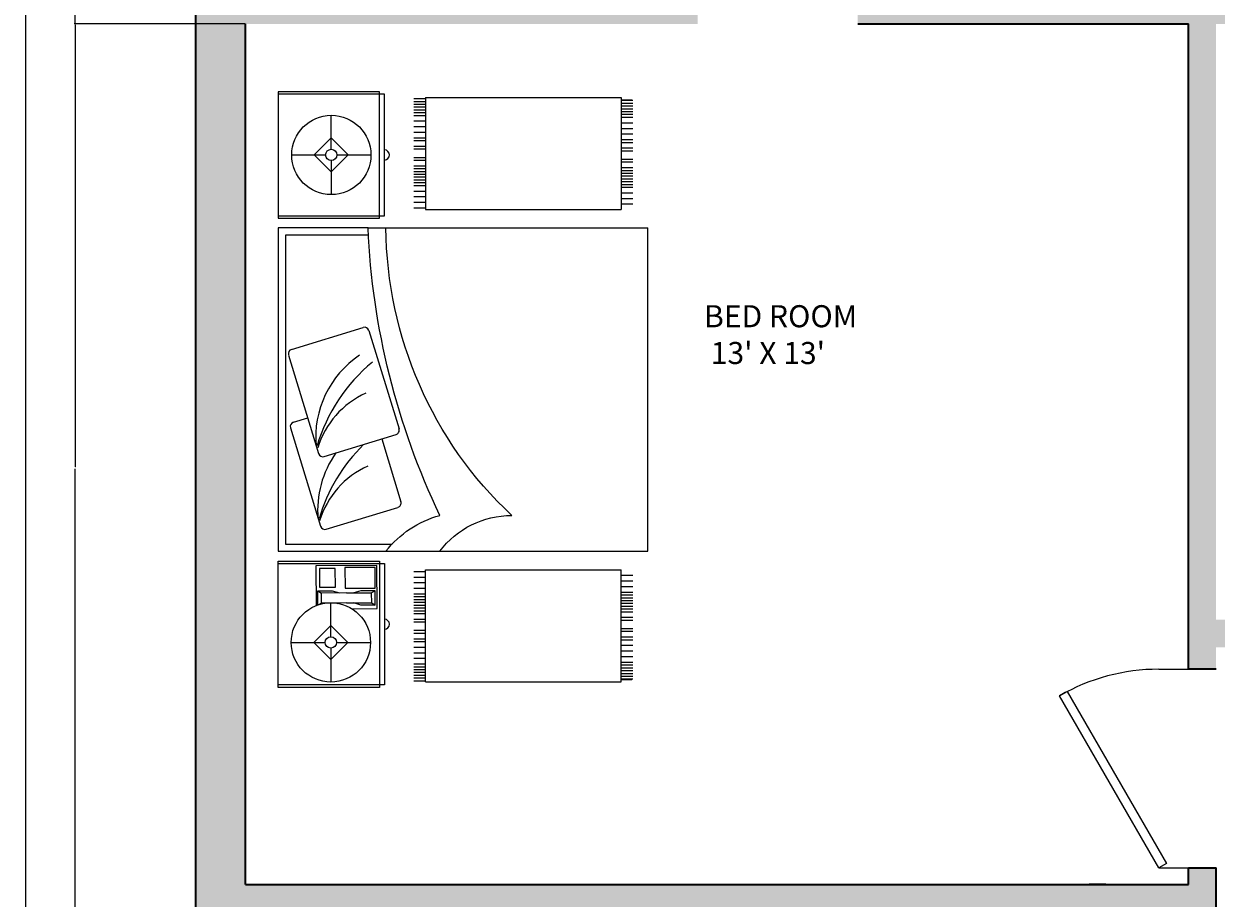
# Model space of a CAD drawing. Units: inches. Extents: x -30 to 437, y -29 to 647.
# Tile 8 of 15: x -30 to 187, y 389 to 548. Entities that reach past the tile are written whole.
import ezdxf

# ---------------------------------------------------------------- set-up
doc = ezdxf.new("R2010")
doc.units = ezdxf.units.IN
doc.header["$MEASUREMENT"] = 0
for name, color, linetype, lineweight in [('A-ANNO-DIMS', 2, 'Continuous', 18), ('A-AREA-IDEN', 7, 'Continuous', 18), ('A-WALL', 7, 'Continuous', 35), ('bedroom', 120, 'Continuous', 18), ('doors', 40, 'Continuous', 25)]:
    doc.layers.add(name, color=color, linetype=linetype, lineweight=lineweight)
doc.layers.add('A-WALL-PATT', color=251, linetype='Continuous', lineweight=13, true_color=0x636466)
doc.styles.get("Standard").update_dxf_attribs({"font": 'arial.ttf'})
doc.dimstyles.get("Standard").update_dxf_attribs({"dimtxt": 0.18, "dimasz": 0.18, "dimexe": 0.18, "dimexo": 0.0625, "dimgap": 0.09, "dimtad": 0, "dimtih": 1, "dimtoh": 1, "dimdec": 4, "dimzin": 0, "dimdsep": 46, "dimtxsty": 'Standard', "dimcen": 0.09, "dimadec": 0, "dimazin": 0, "dimtfac": 1, "dimtdec": 4, "dimtofl": 0, "dimtmove": 0, "dimatfit": 3, "dimfxl": 1, "dimtolj": 1, "dimtzin": 0, "dimarcsym": 0})

# ---------------------------------------------------------------- blocks, each defined once
blk = doc.blocks.new('3')
for p, q in [((185.8665, 224.6766), (185.8665, 225.2363)), ((185.8665, 225.2363), (186.566, 225.2363)), ((185.8805, 224.6487), (185.8805, 225.2363)), ((186.552, 225.2363), (186.552, 224.6487)), ((186.566, 225.2363), (186.566, 224.6766)), ((186.6199, 225.2363), (186.6199, 224.6399)), ((188.4089, 225.2363), (186.6199, 225.2363)), ((188.4089, 224.7393), (188.4089, 225.2363)), ((188.4627, 225.2363), (188.4627, 224.6766)), ((189.1623, 225.2363), (188.4627, 225.2363)), ((188.4767, 225.2363), (188.4767, 224.6486)), ((189.1483, 224.6486), (189.1483, 225.2363)), ((189.1623, 224.6766), (189.1623, 225.2363)), ((186.1157, 225.1643), (186.1157, 224.9763)), ((187.3034, 225.1683), (186.7581, 225.0015)), ((187.7059, 225.1793), (187.1607, 225.0124)), ((187.3344, 225.1518), (187.3586, 225.073)), ((187.737, 225.1628), (187.8585, 224.7657)), ((188.8125, 225.1618), (188.8125, 224.9738)), ((186.0216, 224.9449), (186.1157, 225.0389)), ((186.1157, 225.0389), (186.2097, 224.9449)), ((186.5397, 225.0274), (186.3193, 225.0266)), ((186.3215, 225.0167), (186.4008, 225.017)), ((186.3334, 224.9969), (186.3215, 225.0167)), ((186.3334, 224.9969), (186.389, 224.9971)), ((186.334, 224.858), (186.3334, 224.9969)), ((186.4008, 225.017), (186.389, 224.9971)), ((186.3895, 224.8582), (186.389, 224.9971)), ((186.4008, 225.017), (186.4011, 224.9376)), ((186.5409, 224.6901), (186.5397, 225.0274)), ((188.8125, 225.0365), (188.7185, 224.9424)), ((188.9065, 224.9424), (188.8125, 225.0365)), ((186.0843, 224.9449), (185.8963, 224.9449)), ((186.1157, 224.8509), (186.0216, 224.9449)), ((186.2097, 224.9449), (186.1157, 224.8509)), ((186.147, 224.9449), (186.335, 224.9449)), ((186.4011, 224.9376), (186.3894, 224.8979)), ((186.7416, 224.9704), (186.8631, 224.5734)), ((187.1442, 224.9814), (187.2657, 224.5843)), ((188.7812, 224.9424), (188.5931, 224.9424)), ((188.7185, 224.9424), (188.8125, 224.8484)), ((188.8125, 224.8484), (188.9065, 224.9424)), ((188.8438, 224.9424), (189.0319, 224.9424)), ((186.1157, 224.9136), (186.1157, 224.7256)), ((186.3314, 224.9055), (186.3338, 224.8977)), ((186.334, 224.858), (186.3345, 224.7191)), ((186.3895, 224.8582), (186.39, 224.7193)), ((188.8125, 224.9111), (188.8125, 224.723)), ((186.3023, 224.8297), (186.3029, 224.6892)), ((186.3224, 224.7786), (186.3341, 224.8183)), ((186.4017, 224.7789), (186.3897, 224.8185)), ((186.3227, 224.6992), (186.3224, 224.7786)), ((186.402, 224.6995), (186.4017, 224.7789)), ((187.842, 224.7347), (187.2967, 224.5678)), ((188.4089, 224.7393), (188.4089, 223.1907)), ((186.566, 224.6766), (185.8665, 224.6766)), ((186.3029, 224.6892), (186.5409, 224.6901)), ((186.3345, 224.7191), (186.3227, 224.6992)), ((186.3227, 224.6992), (186.402, 224.6995)), ((186.3345, 224.7191), (186.39, 224.7193)), ((186.402, 224.6995), (186.39, 224.7193)), ((187.2416, 224.6632), (186.8942, 224.5569)), ((188.4627, 224.6766), (189.1623, 224.6766)), ((186.552, 224.6487), (185.8805, 224.6487)), ((186.6199, 224.6399), (186.6199, 223.1907)), ((188.4767, 224.6486), (189.1483, 224.6486)), ((185.904, 224.4849, -0.9094), (185.904, 224.4204, -0.9094)), ((185.9195, 224.4849, -0.9094), (185.9195, 224.4204, -0.9094)), ((185.9195, 224.4849, -0.9094), (185.9195, 224.4204, -0.9094)), ((185.935, 224.4849, -0.9094), (185.935, 224.4204, -0.9094)), ((185.9505, 224.4849, -0.9094), (185.9505, 224.4204, -0.9094)), ((185.966, 224.4849, -0.9094), (185.966, 224.4204, -0.9094)), ((185.9815, 224.4849, -0.9094), (185.9815, 224.4204, -0.9094)), ((185.997, 224.4849, -0.9094), (185.997, 224.4204, -0.9094)), ((186.028, 224.4849, -0.9094), (186.028, 224.4204, -0.9094)), ((186.059, 224.4849, -0.9094), (186.059, 224.4204, -0.9094)), ((186.09, 224.4849, -0.9094), (186.09, 224.4204, -0.9094)), ((186.09, 224.4849, -0.9094), (186.09, 224.4204, -0.9094)), ((186.121, 224.4849, -0.9094), (186.121, 224.4204, -0.9094)), ((186.1365, 224.4849, -0.9094), (186.1365, 224.4204, -0.9094)), ((186.1675, 224.4849, -0.9094), (186.1675, 224.4204, -0.9094)), ((186.183, 224.4849, -0.9094), (186.183, 224.4204, -0.9094)), ((186.2295, 224.4849, -0.9094), (186.2295, 224.4204, -0.9094)), ((186.245, 224.4849, -0.9094), (186.245, 224.4204, -0.9094)), ((186.276, 224.4849, -0.9094), (186.276, 224.4204, -0.9094)), ((186.2915, 224.4849, -0.9094), (186.2915, 224.4204, -0.9094)), ((186.307, 224.4849, -0.9094), (186.307, 224.4204, -0.9094)), ((186.3225, 224.4849, -0.9094), (186.3225, 224.4204, -0.9094)), ((186.338, 224.4849, -0.9094), (186.338, 224.4204, -0.9094)), ((186.3535, 224.4849, -0.9094), (186.3535, 224.4204, -0.9094)), ((186.369, 224.4849, -0.9094), (186.369, 224.4204, -0.9094)), ((186.3845, 224.4849, -0.9094), (186.3845, 224.4204, -0.9094)), ((186.4155, 224.4849, -0.9094), (186.4155, 224.4204, -0.9094)), ((186.4465, 224.4849, -0.9094), (186.4465, 224.4204, -0.9094)), ((186.4775, 224.4849, -0.9094), (186.4775, 224.4204, -0.9094)), ((186.5085, 224.4849, -0.9094), (186.5085, 224.4204, -0.9094)), ((188.5202, 224.4849, -0.9094), (188.5202, 224.4204, -0.9094)), ((188.5512, 224.4849, -0.9094), (188.5512, 224.4204, -0.9094)), ((188.5822, 224.4849, -0.9094), (188.5822, 224.4204, -0.9094)), ((188.6132, 224.4849, -0.9094), (188.6132, 224.4204, -0.9094)), ((188.6442, 224.4849, -0.9094), (188.6442, 224.4204, -0.9094)), ((188.6597, 224.4849, -0.9094), (188.6597, 224.4204, -0.9094)), ((188.6752, 224.4849, -0.9094), (188.6752, 224.4204, -0.9094)), ((188.6907, 224.4849, -0.9094), (188.6907, 224.4204, -0.9094)), ((188.7062, 224.4849, -0.9094), (188.7062, 224.4204, -0.9094)), ((188.7217, 224.4849, -0.9094), (188.7217, 224.4204, -0.9094)), ((188.7372, 224.4849, -0.9094), (188.7372, 224.4204, -0.9094)), ((188.7527, 224.4849, -0.9094), (188.7527, 224.4204, -0.9094)), ((188.7837, 224.4849, -0.9094), (188.7837, 224.4204, -0.9094)), ((188.7992, 224.4849, -0.9094), (188.7992, 224.4204, -0.9094)), ((188.8457, 224.4849, -0.9094), (188.8457, 224.4204, -0.9094)), ((188.8612, 224.4849, -0.9094), (188.8612, 224.4204, -0.9094)), ((188.8922, 224.4849, -0.9094), (188.8922, 224.4204, -0.9094)), ((188.9077, 224.4849, -0.9094), (188.9077, 224.4204, -0.9094)), ((188.9387, 224.4849, -0.9094), (188.9387, 224.4204, -0.9094)), ((188.9387, 224.4849, -0.9094), (188.9387, 224.4204, -0.9094)), ((188.9697, 224.4849, -0.9094), (188.9697, 224.4204, -0.9094)), ((189.0007, 224.4849, -0.9094), (189.0007, 224.4204, -0.9094)), ((189.0317, 224.4849, -0.9094), (189.0317, 224.4204, -0.9094)), ((189.0472, 224.4849, -0.9094), (189.0472, 224.4204, -0.9094)), ((189.0627, 224.4849, -0.9094), (189.0627, 224.4204, -0.9094)), ((189.0782, 224.4849, -0.9094), (189.0782, 224.4204, -0.9094)), ((189.0937, 224.4849, -0.9094), (189.0937, 224.4204, -0.9094)), ((189.1092, 224.4849, -0.9094), (189.1092, 224.4204, -0.9094)), ((189.1092, 224.4849, -0.9094), (189.1092, 224.4204, -0.9094)), ((189.1247, 224.4849, -0.9094), (189.1247, 224.4204, -0.9094)), ((185.8974, 224.4204, -0.9094), (185.8974, 223.3378, -0.9094)), ((185.8974, 224.4204, -0.9094), (186.5174, 224.4204, -0.9094)), ((186.5174, 224.4204, -0.9094), (186.5174, 223.3378, -0.9094)), ((189.1313, 224.4204, -0.9094), (188.5113, 224.4204, -0.9094)), ((188.5113, 224.4204, -0.9094), (188.5113, 223.3378, -0.9094)), ((189.1313, 224.4204, -0.9094), (189.1313, 223.3378, -0.9094)), ((185.8974, 223.3378, -0.9094), (186.5174, 223.3378, -0.9094)), ((185.9114, 223.3378, -0.9094), (185.9114, 223.2789, -0.9094)), ((185.9114, 223.3378, -0.9094), (185.9114, 223.2789, -0.9094)), ((185.9114, 223.3378, -0.9094), (185.9114, 223.2789, -0.9094)), ((185.9138, 223.3378, -0.9094), (185.9138, 223.2732, -0.9094)), ((185.9293, 223.3378, -0.9094), (185.9293, 223.2732, -0.9094)), ((185.9293, 223.3378, -0.9094), (185.9293, 223.2732, -0.9094)), ((185.9448, 223.3378, -0.9094), (185.9448, 223.2732, -0.9094)), ((185.9603, 223.3378, -0.9094), (185.9603, 223.2732, -0.9094)), ((185.9758, 223.3378, -0.9094), (185.9758, 223.2732, -0.9094)), ((185.9913, 223.3378, -0.9094), (185.9913, 223.2732, -0.9094)), ((186.0068, 223.3378, -0.9094), (186.0068, 223.2732, -0.9094)), ((186.0378, 223.3378, -0.9094), (186.0378, 223.2732, -0.9094)), ((186.0688, 223.3378, -0.9094), (186.0688, 223.2732, -0.9094)), ((186.0998, 223.3378, -0.9094), (186.0998, 223.2732, -0.9094)), ((186.0998, 223.3378, -0.9094), (186.0998, 223.2732, -0.9094)), ((186.1308, 223.3378, -0.9094), (186.1308, 223.2732, -0.9094)), ((186.1463, 223.3378, -0.9094), (186.1463, 223.2732, -0.9094)), ((186.1773, 223.3378, -0.9094), (186.1773, 223.2732, -0.9094)), ((186.1928, 223.3378, -0.9094), (186.1928, 223.2732, -0.9094)), ((186.2393, 223.3378, -0.9094), (186.2393, 223.2732, -0.9094)), ((186.2548, 223.3378, -0.9094), (186.2548, 223.2732, -0.9094)), ((186.2858, 223.3378, -0.9094), (186.2858, 223.2732, -0.9094)), ((186.3013, 223.3378, -0.9094), (186.3013, 223.2732, -0.9094)), ((186.3168, 223.3378, -0.9094), (186.3168, 223.2732, -0.9094)), ((186.3323, 223.3378, -0.9094), (186.3323, 223.2732, -0.9094)), ((186.3478, 223.3378, -0.9094), (186.3478, 223.2732, -0.9094)), ((186.3633, 223.3378, -0.9094), (186.3633, 223.2732, -0.9094)), ((186.3788, 223.3378, -0.9094), (186.3788, 223.2732, -0.9094)), ((186.3943, 223.3378, -0.9094), (186.3943, 223.2732, -0.9094)), ((186.4253, 223.3378, -0.9094), (186.4253, 223.2732, -0.9094)), ((186.4563, 223.3378, -0.9094), (186.4563, 223.2732, -0.9094)), ((186.4873, 223.3378, -0.9094), (186.4873, 223.2732, -0.9094)), ((189.1313, 223.3378, -0.9094), (188.5113, 223.3378, -0.9094)), ((188.5414, 223.3378, -0.9094), (188.5414, 223.2732, -0.9094)), ((188.5724, 223.3378, -0.9094), (188.5724, 223.2732, -0.9094)), ((188.6034, 223.3378, -0.9094), (188.6034, 223.2732, -0.9094)), ((188.6344, 223.3378, -0.9094), (188.6344, 223.2732, -0.9094)), ((188.6499, 223.3378, -0.9094), (188.6499, 223.2732, -0.9094)), ((188.6654, 223.3378, -0.9094), (188.6654, 223.2732, -0.9094)), ((188.6809, 223.3378, -0.9094), (188.6809, 223.2732, -0.9094)), ((188.6964, 223.3378, -0.9094), (188.6964, 223.2732, -0.9094)), ((188.7119, 223.3378, -0.9094), (188.7119, 223.2732, -0.9094)), ((188.7274, 223.3378, -0.9094), (188.7274, 223.2732, -0.9094)), ((188.7429, 223.3378, -0.9094), (188.7429, 223.2732, -0.9094)), ((188.7739, 223.3378, -0.9094), (188.7739, 223.2732, -0.9094)), ((188.7894, 223.3378, -0.9094), (188.7894, 223.2732, -0.9094)), ((188.8359, 223.3378, -0.9094), (188.8359, 223.2732, -0.9094)), ((188.8514, 223.3378, -0.9094), (188.8514, 223.2732, -0.9094)), ((188.8824, 223.3378, -0.9094), (188.8824, 223.2732, -0.9094)), ((188.8979, 223.3378, -0.9094), (188.8979, 223.2732, -0.9094)), ((188.9289, 223.3378, -0.9094), (188.9289, 223.2732, -0.9094)), ((188.9289, 223.3378, -0.9094), (188.9289, 223.2732, -0.9094)), ((188.9599, 223.3378, -0.9094), (188.9599, 223.2732, -0.9094)), ((188.9909, 223.3378, -0.9094), (188.9909, 223.2732, -0.9094)), ((189.022, 223.3378, -0.9094), (189.022, 223.2732, -0.9094)), ((189.0375, 223.3378, -0.9094), (189.0375, 223.2732, -0.9094)), ((189.053, 223.3378, -0.9094), (189.053, 223.2732, -0.9094)), ((189.0685, 223.3378, -0.9094), (189.0685, 223.2732, -0.9094)), ((189.084, 223.3378, -0.9094), (189.084, 223.2732, -0.9094)), ((189.0995, 223.3378, -0.9094), (189.0995, 223.2732, -0.9094)), ((189.0995, 223.3378, -0.9094), (189.0995, 223.2732, -0.9094)), ((189.115, 223.3378, -0.9094), (189.115, 223.2732, -0.9094)), ((189.1173, 223.3378, -0.9094), (189.1173, 223.2789, -0.9094)), ((189.1173, 223.3378, -0.9094), (189.1173, 223.2789, -0.9094)), ((189.1173, 223.3378, -0.9094), (189.1173, 223.2789, -0.9094)), ((186.6199, 223.1907), (188.4089, 223.1907))]:
    blk.add_line(p, q)
blk.add_lwpolyline([(188.3691, 224.7374), (188.3691, 225.1965), (186.6596, 225.1965), (186.6596, 224.606)])
for points in [[(186.4217, 225.0072), (186.422, 224.9199), (186.5252, 224.9202), (186.5249, 225.0075)], [(186.4153, 224.8663), (186.4159, 224.6996), (186.531, 224.7), (186.5304, 224.8667)]]:
    blk.add_lwpolyline(points, close=True)
for points in [[(186.6199, 224.6399, -0.162278), (186.8186, 224.3418, -0.100664), (188.4089, 224.7393, -0.100664)], [(186.6199, 224.3418, -0.236068), (186.8186, 223.9442, -0.205258), (188.4089, 224.6399, -0.205258)]]:
    blk.add_lwpolyline(points, format="xyb")
for centre, radius in [((186.1157, 224.9449), 0.2194), ((188.8125, 224.9424), 0.2194), ((186.1157, 224.9449), 0.0313), ((188.8125, 224.9424), 0.0313)]:
    blk.add_circle(centre, radius)
for centre, radius, start, end in [((187.3107, 225.1446), 0.0248, 17.0142, 107.0142), ((187.7132, 225.1555), 0.0248, 17.0142, 107.0142), ((186.7654, 224.9777), 0.0248, 107.0142, 197.0142), ((186.6474, 224.5408), 0.4873, 24.22087, 73.06906), ((186.8477, 224.4712), 0.5468, 54.68511, 95.16051), ((186.5359, 224.1054), 0.9426, 44.27274, 73.71889), ((187.1679, 224.9887), 0.0248, 107.0142, 197.0142), ((187.0499, 224.5517), 0.4873, 24.22087, 73.06906), ((187.2502, 224.4821), 0.5468, 33.78007, 95.16051), ((186.9385, 224.1164), 0.9426, 39.40233, 73.71889), ((187.8347, 224.7585), 0.0248, 287.0142, 17.0142), ((186.2163, 224.6487), 0.028, 180, 0), ((188.8125, 224.6486), 0.028, 180, 0), ((186.8869, 224.5806), 0.0248, 197.0142, 287.0142), ((187.2894, 224.5916), 0.0248, 197.0142, 287.0142)]:
    blk.add_arc(centre, radius, start, end)
blk = doc.blocks.new('*U6')
for p, q in [((0, 0), (0, -6)), ((40, 0), (40, -6))]:
    blk.add_line(p, q)
blk.add_lwpolyline([(0, 0), (34.64, 20), (35.52, 18.48), (0.87, -1.52)], close=True)
blk.add_arc((0, 0), 40, 0, 30)
blk = doc.blocks.new('*D26')
at = {"layer": 'A-ANNO-DIMS', "color": 0, "lineweight": -2, "transparency": 16777216}
for p, q in [((1.61, 615.55), (-29.41, 615.55)), ((-29.23, 615.37), (-29.23, 308.98)), ((-29.23, 2.23), (-29.23, 308.62)), ((1.61, 2.05), (-29.41, 2.05))]:
    blk.add_line(p, q, dxfattribs=at)
at = {"layer": 'A-ANNO-DIMS', "color": 0, "transparency": 16777216}
for points in [[(-29.26, 615.37), (-29.2, 615.37), (-29.23, 615.55)], [(-29.26, 2.23), (-29.2, 2.23), (-29.23, 2.05)]]:
    blk.add_solid(points, dxfattribs=at)
at = {"layer": 'Defpoints', "color": 0, "transparency": 16777216}
for p in [(-29.23, 615.55), (1.67, 615.55), (1.67, 2.05)]:
    blk.add_point(p, dxfattribs=at)
at = {"layer": 'A-ANNO-DIMS', "color": 0, "transparency": 16777216, "insert": (-29.23, 308.8), "char_height": 0.18, "attachment_point": 5}
blk.add_mtext('\\A1;613.5', dxfattribs=at)
blk = doc.blocks.new('*D33')
at = {"layer": 'A-ANNO-DIMS', "color": 0, "lineweight": -2, "transparency": 16777216}
for p, q in [((10.61, 547.55), (-20.41, 547.55)), ((-20.23, 547.37), (-20.23, 467.23)), ((-20.23, 386.73), (-20.23, 466.87)), ((10.61, 386.55), (-20.41, 386.55))]:
    blk.add_line(p, q, dxfattribs=at)
at = {"layer": 'A-ANNO-DIMS', "color": 0, "transparency": 16777216}
for points in [[(-20.26, 547.37), (-20.2, 547.37), (-20.23, 547.55)], [(-20.26, 386.73), (-20.2, 386.73), (-20.23, 386.55)]]:
    blk.add_solid(points, dxfattribs=at)
at = {"layer": 'Defpoints', "color": 0, "transparency": 16777216}
for p in [(-20.23, 547.55), (10.67, 547.55), (10.67, 386.55)]:
    blk.add_point(p, dxfattribs=at)
at = {"layer": 'A-ANNO-DIMS', "color": 0, "transparency": 16777216, "insert": (-20.23, 467.05), "char_height": 0.18, "attachment_point": 5}
blk.add_mtext('\\A1;161', dxfattribs=at)
blk = doc.blocks.new('*D34')
at = {"layer": 'A-ANNO-DIMS', "color": 0, "lineweight": -2, "transparency": 16777216}
for p, q in [((10.61, 606.55), (-20.41, 606.55)), ((-20.23, 606.37), (-20.23, 577.23)), ((-20.23, 547.73), (-20.23, 576.87)), ((10.61, 547.55), (-20.41, 547.55))]:
    blk.add_line(p, q, dxfattribs=at)
at = {"layer": 'A-ANNO-DIMS', "color": 0, "transparency": 16777216}
for points in [[(-20.26, 606.37), (-20.2, 606.37), (-20.23, 606.55)], [(-20.26, 547.73), (-20.2, 547.73), (-20.23, 547.55)]]:
    blk.add_solid(points, dxfattribs=at)
at = {"layer": 'Defpoints', "color": 0, "transparency": 16777216}
for p in [(-20.23, 606.55), (10.67, 606.55), (10.67, 547.55)]:
    blk.add_point(p, dxfattribs=at)
at = {"layer": 'A-ANNO-DIMS', "color": 0, "transparency": 16777216, "insert": (-20.23, 577.05), "char_height": 0.18, "attachment_point": 5}
blk.add_mtext('\\A1;59', dxfattribs=at)

msp = doc.modelspace()

# ---------------------------------------------------------------- hatches: boundary and pattern name
at = {"layer": 'A-WALL-PATT'}
h = msp.add_hatch(color=256, dxfattribs=at)
h.dxf.hatch_style = 1
h.paths.add_polyline_path([(393.6054, 183.2352), (369.6054, 183.2352), (369.6054, 213.2352), (393.6054, 213.2352), (393.6054, 207.2352), (394.6054, 207.2352), (394.6054, 211.2352), (395.6054, 211.2352), (395.6054, 185.2352), (394.6054, 185.2352), (394.6054, 189.2352), (393.6054, 189.2352)], flags=0)
h.paths.add_polyline_path([(384.6054, 189.2352, -1), (390.6054, 189.2352, -1)], flags=0)
h.paths.add_polyline_path([(385.6054, 189.2352, -1), (389.6054, 189.2352, -1)], flags=0)
h.paths.add_polyline_path([(374.6054, 189.2352, -1), (382.6054, 189.2352, -1)], flags=0)
h.paths.add_polyline_path([(386.6054, 189.2352, -1), (388.6054, 189.2352, -1)], flags=0)
h.paths.add_polyline_path([(375.6054, 189.2352, -1), (381.6054, 189.2352, -1)], flags=0)
h.paths.add_polyline_path([(376.6054, 189.2352, -1), (380.6054, 189.2352, -1)], flags=0)
h.paths.add_polyline_path([(377.6054, 189.2352, -1), (379.6054, 189.2352, -1)], flags=0)
h.paths.add_polyline_path([(390.6054, 195.2352), (374.6054, 195.2352), (374.6054, 201.2352), (390.6054, 201.2352)], flags=0)
h.paths.add_polyline_path([(389.6054, 196.2352), (375.6054, 196.2352), (375.6054, 200.2352), (389.6054, 200.2352)], flags=0)
h.paths.add_polyline_path([(383.6054, 207.2352, -1), (391.6054, 207.2352, -1)], flags=0)
h.paths.add_polyline_path([(384.6054, 207.2352, -1), (390.6054, 207.2352, -1)], flags=0)
h.paths.add_polyline_path([(385.6054, 207.2352, -1), (389.6054, 207.2352, -1)], flags=0)
h.paths.add_polyline_path([(386.6054, 207.2352, -1), (388.6054, 207.2352, -1)], flags=0)
h.paths.add_polyline_path([(375.6054, 207.2352, -1), (381.6054, 207.2352, -1)], flags=0)
h.paths.add_polyline_path([(376.6054, 207.2352, -1), (380.6054, 207.2352, -1)], flags=0)
h.paths.add_polyline_path([(377.6054, 207.2352, -1), (379.6054, 207.2352, -1)], flags=0)
h.paths.add_polyline_path([(305.5437, 160.3663, -0.41421356), (304.0437, 158.8663), (271.0437, 158.8663, -0.41421356), (269.5437, 160.3663), (269.5437, 178.3663, -0.41421356), (271.0437, 179.8663), (304.0437, 179.8663, -0.41421356), (305.5437, 178.3663)], flags=0)
h.paths.add_polyline_path([(304.0437, 165.3663, -0.41421356), (303.0437, 164.3663), (289.2937, 164.3663, -0.41421356), (288.2937, 165.3663), (288.2937, 177.3663, -0.41421356), (289.2937, 178.3663), (303.0437, 178.3663, -0.41421356), (304.0437, 177.3663)], flags=0)
h.paths.add_polyline_path([(296.5437, 171.3663, -1), (295.5437, 171.3663, -1)], flags=0)
h.paths.add_polyline_path([(286.7937, 165.3663, -0.41421356), (285.7937, 164.3663), (272.0437, 164.3663, -0.41421356), (271.0437, 165.3663), (271.0437, 177.3663, -0.41421356), (272.0437, 178.3663), (285.7937, 178.3663, -0.41421356), (286.7937, 177.3663)], flags=0)
h.paths.add_polyline_path([(279.5437, 171.3663, -1), (278.5437, 171.3663, -1)], flags=0)
h.paths.add_polyline_path([(360.6737, 290.5474), (360.6737, 300.5474), (396.6737, 300.5474), (396.6737, 290.5474)], flags=0)
h.paths.add_polyline_path([(259.6737, 124.5474), (259.6737, 114.5474), (171.6737, 114.5474), (171.6737, 124.5474)], flags=0)
h.paths.add_polyline_path([(288.0737, 215.3705), (286.7097, 214.583), (268.7097, 245.7599), (270.0737, 246.5474)], flags=0)
h.paths.add_polyline_path([(259.6737, 168.5474), (256.6737, 168.5474), (256.6737, 173.5474), (256.6737, 179.0224), (255.8753, 177.6395), (224.2956, 195.872, 0.12053744), (220.1737, 179.0224, 0.12053744), (216.0518, 195.872), (184.4721, 177.6395), (183.6737, 179.0224), (215.2836, 197.2724), (216.0821, 195.8895), (216.0518, 195.872, -0.12053744), (220.1737, 179.0224, -0.12053744), (224.2956, 195.872), (224.2653, 195.8895), (225.0638, 197.2724), (256.6737, 179.0224), (256.6737, 173.5474), (259.6737, 173.5474)], flags=0)
h.paths.add_polyline_path([(386.7943, 325.4601), (372.6871, 325.4601), (372.6871, 339.5673), (386.7943, 339.5673)], flags=0)
h.paths.add_polyline_path([(359.5875, 343.7429), (357.7905, 343.7429), (357.7905, 327.9179), (359.3933, 327.9179, 0.41420885), (361.5302, 330.0549), (361.5302, 341.8434, 0.41436161)], flags=0)
h.paths.add_polyline_path([(341.7887, 323.1235, -0.11921667), (340.7839, 323.1235)], flags=0)
h.paths.add_polyline_path([(379.6332, 328.8632), (379.6332, 332.2699), (376.0992, 332.2699, 0.39427733)], flags=0)
h.paths.add_polyline_path([(375.5299, 332.459, -1), (383.8511, 332.459, -1)], flags=0)
h.paths.add_polyline_path([(388.9363, 344.7425), (372.5309, 344.7425, -0.41421356), (370.394, 346.8794), (370.394, 347.5594, -0.39085173), (372.3472, 349.7005, -0.43951011), (370.394, 351.4933), (370.394, 365.1894, -0.40305452), (372.2191, 367.1298, -0.41839453), (370.394, 368.9291), (370.394, 382.6251, -0.40885826), (372.2519, 384.5722, -0.42377324), (370.394, 386.3707), (370.394, 400.0667, -0.38660687), (372.1327, 402.0094), (372.531, 402.0094, -0.41421834), (370.394, 404.1464), (370.394, 404.7778, -0.41420891), (372.5309, 406.9147), (388.9363, 406.9147, -0.41421821), (391.0733, 404.7778), (391.0733, 346.8794, -0.41421356)], flags=0)
edge = h.paths.add_edge_path(flags=0)
edge.add_spline(control_points=[(349.3585, 363.204), (349.0859, 363.204), (348.8133, 363.2227), (348.2712, 363.2973), (348.0016, 363.3531), (347.3533, 363.5328), (346.9776, 363.6755), (346.2445, 364.0308), (345.887, 364.2432), (345.1953, 364.7329), (344.8611, 365.0101), (344.2197, 365.6237), (343.9125, 365.9603), (343.211, 366.8336), (342.8313, 367.3965), (342.1401, 368.6117), (341.8286, 369.2641), (341.2807, 370.64), (341.0443, 371.3636), (340.6522, 372.8619), (340.4964, 373.6367), (340.2695, 375.2158), (340.1983, 376.0203), (340.142, 377.6365), (340.157, 378.4483), (340.2729, 380.0567), (340.3738, 380.8533), (340.6589, 382.4093), (340.8432, 383.1686), (341.2906, 384.629), (341.5538, 385.3301), (342.1531, 386.6544), (342.4891, 387.2776), (343.2266, 388.4288), (343.6281, 388.9567), (344.4879, 389.9012), (344.9463, 390.3178), (345.7981, 390.9428), (346.182, 391.1771), (346.9712, 391.5648), (347.3766, 391.7182), (348.2004, 391.9387), (348.6189, 392.0058), (349.4588, 392.0508), (349.8801, 392.0288), (350.7146, 391.8966), (351.1278, 391.7865), (351.9366, 391.4822), (352.3323, 391.2882), (353.0989, 390.8223), (353.4699, 390.5504), (354.1819, 389.9355), (354.5229, 389.5924), (355.1706, 388.8418), (355.4772, 388.4343), (356.1315, 387.4422), (356.4671, 386.8397), (357.0692, 385.5581), (357.3356, 384.879), (357.7933, 383.4624), (357.9846, 382.725), (358.2875, 381.2112), (358.3992, 380.4349), (358.5404, 378.8643), (358.5699, 378.0699), (358.546, 376.4841), (358.4926, 375.6928), (358.3042, 374.1343), (358.1692, 373.3672), (357.8207, 371.8774), (357.6072, 371.1549), (357.1067, 369.7735), (356.8196, 369.1148), (356.1782, 367.8787), (355.8238, 367.3013), (355.0551, 366.244), (354.6408, 365.7641), (353.7607, 364.9161), (353.2948, 364.5481), (352.445, 364.0149), (352.0701, 363.822), (351.3034, 363.5117), (350.9116, 363.3943), (350.1325, 363.2418), (349.7455, 363.204), (349.3585, 363.204)], knot_values=[3.14159265, 3.14159265, 3.14159265, 3.14159265, 3.22691715, 3.22691715, 3.31224165, 3.31224165, 3.43426671, 3.43426671, 3.55629177, 3.55629177, 3.67831683, 3.67831683, 3.8003419, 3.8003419, 3.97157384, 3.97157384, 4.14280577, 4.14280577, 4.31403771, 4.31403771, 4.48526965, 4.48526965, 4.65650159, 4.65650159, 4.82773353, 4.82773353, 4.99896547, 4.99896547, 5.1701974, 5.1701974, 5.34142934, 5.34142934, 5.51266128, 5.51266128, 5.68389322, 5.68389322, 5.85512516, 5.85512516, 5.98669107, 5.98669107, 6.11825699, 6.11825699, 6.24982291, 6.24982291, 6.38138882, 6.38138882, 6.51295474, 6.51295474, 6.64452065, 6.64452065, 6.77608657, 6.77608657, 6.90765249, 6.90765249, 7.0392184, 7.0392184, 7.20701563, 7.20701563, 7.37481286, 7.37481286, 7.54261009, 7.54261009, 7.71040732, 7.71040732, 7.87820455, 7.87820455, 8.04600178, 8.04600178, 8.21379901, 8.21379901, 8.38159624, 8.38159624, 8.54939347, 8.54939347, 8.7171907, 8.7171907, 8.88498794, 8.88498794, 9.05278517, 9.05278517, 9.17820699, 9.17820699, 9.30362881, 9.30362881, 9.42477796, 9.42477796, 9.42477796, 9.42477796], degree=3, periodic=0)
edge.add_line((341.1696, 384.3006), (341.2012, 384.2808))
edge = h.paths.add_edge_path(flags=0)
edge.add_line((344.3353, 388.7801), (344.317, 388.7915))
edge.add_ellipse((349.3585, 377.6204), major_axis=(0, -13.7895), ratio=0.62186025, start_angle=-244.867444, end_angle=-124.769923)
h.paths.add_polyline_path([(163.6737, 163.1474), (132.4968, 145.1474), (131.7093, 146.5114), (162.8862, 164.5114)], flags=0)
h.paths.add_polyline_path([(366.4355, 409.0896, -0.41423669), (364.2985, 406.9525, -0.4913499), (361.5302, 408.8973), (361.5302, 420.6405, 0.41421356), (359.3932, 422.7775), (357.7905, 422.7775), (357.7905, 406.9525), (359.6317, 406.9525, 0.42741026), (361.5332, 408.9757, 0.39869469), (363.6672, 406.9525, 0.51958103), (366.4355, 409.0895)], flags=0)
h.paths.add_polyline_path([(386.7943, 410.9671), (372.6871, 410.9671), (372.6871, 425.0742), (386.7943, 425.0742)], flags=0)
h.paths.add_polyline_path([(379.6332, 414.3701), (379.6332, 417.7768), (376.0992, 417.7768, 0.39427733)], flags=0)
h.paths.add_polyline_path([(375.5299, 417.966, -1), (383.8511, 417.966, -1)], flags=0)
h.paths.add_polyline_path([(150.0377, 351.583), (148.6737, 352.3705), (166.6737, 383.5474), (168.0377, 382.7599)], flags=0)
h.paths.add_polyline_path([(91.6737, 234.1974), (66.559, 219.6974), (65.9246, 220.7962), (91.0393, 235.2962)], flags=0)
h.paths.add_polyline_path([(255.4612, 443.5834), (254.6737, 444.9474), (285.8506, 462.9474), (286.6381, 461.5834)], flags=0)
h.paths.add_polyline_path([(176.2737, 394.5474), (158.2737, 425.7243), (159.6377, 426.5118), (177.6377, 395.3349)], flags=0)
h.paths.add_polyline_path([(243.6737, 439.5474), (243.0393, 438.4486), (217.9246, 452.9486), (218.559, 454.0474)], flags=0)
h.paths.add_polyline_path([(38.1264, 269.8429), (40.2408, 269.8429), (40.2408, 270.3508), (38.1264, 270.3508)], flags=0)
h.paths.add_polyline_path([(75.7157, 289.9439), (40.2408, 289.9439), (38.1264, 289.6524), (40.2408, 289.6524)], flags=0)
h.paths.add_polyline_path([(75.7157, 270.0846), (77.6447, 270.0846), (77.6697, 270.1626), (75.7175, 270.1626)], flags=0)
h.paths.add_polyline_path([(80.5373, 293.3002), (33.0467, 293.3002), (13.5054, 293.3002), (13.5054, 351.9244), (29.7898, 351.9244), (80.5373, 351.9244)], flags=0)
h.paths.add_polyline_path([(46.0261, 212.466, -0.50131678), (27.1651, 207.5106), (21.165, 209.5107), (21.165, 206.5107), (22.665, 206.5107), (22.665, 203.5107), (21.165, 203.5107), (21.165, 203.0107), (13.165, 203.0107), (13.165, 224.0107), (21.165, 224.0107), (21.165, 217.5107), (27.1649, 219.5106, -0.50132349), (46.0261, 214.5554, -0.13289091)], flags=0)
h.paths.add_polyline_path([(44.688, 211.8666, -0.48007965), (27.165, 209.5107), (27.165, 217.5107, -0.4800795), (44.688, 215.1547, -0.21500378)], flags=0)
h.paths.add_polyline_path([(19.415, 204.0107), (15.165, 204.0107, -0.41421356), (14.165, 204.7607), (14.165, 222.0107, -0.41421356), (14.915, 223.0107), (19.165, 223.0107, -0.41421356), (20.165, 222.2607), (20.165, 205.0107, -0.41421356)], flags=0)
h.paths.add_polyline_path([(32.7608, 269.0719), (31.8439, 269.0719), (31.8439, 268.6134), (13.5054, 268.6134), (13.5054, 291.5366), (31.8439, 291.5366), (32.7608, 291.0781), (32.7608, 280.9919, -1), (32.7608, 279.1581)], flags=0)
h.paths.add_polyline_path([(40.2408, 360.1436), (38.1264, 360.1436), (38.1264, 359.6357), (40.2408, 359.6357)], flags=0)
h.paths.add_polyline_path([(75.7157, 355.2807), (40.2408, 355.2807), (38.1264, 355.5722), (40.2408, 355.5722), (40.2408, 355.2807), (75.7157, 355.2807), (75.7157, 375.5982), (40.2408, 375.5982), (38.1264, 375.3817), (40.2408, 375.3817), (40.2408, 375.5982), (75.7157, 375.5982), (77.9733, 375.062), (75.7175, 375.062), (75.7175, 374.554)], flags=0)
h.paths.add_polyline_path([(42.8174, 299.814, 0.13867074), (34.1602, 294.603), (14.8081, 294.603), (14.8081, 350.6216), (29.8539, 350.6216, 0.09822056)], flags=0)
h.paths.add_polyline_path([(15.8636, 276.7781, -0.30640166), (20.3757, 283.4499), (20.3483, 290.6726), (31.4014, 290.7146), (31.4309, 282.9124), (26.8287, 282.895, -0.26006276), (30.241, 276.7781, -1)], flags=0)
h.paths.add_polyline_path([(26.1332, 276.7781), (23.0523, 273.6972), (19.9714, 276.7781), (23.0523, 279.8589), (23.0523, 283.9209), (21.3493, 283.9145), (20.7006, 283.5219), (20.6907, 286.1226), (23.2914, 286.1325), (25.8936, 285.7522), (27.1939, 285.7572), (28.4928, 286.1522), (31.0935, 286.1621), (31.0918, 286.6172), (25.6303, 286.5965), (25.616, 290.3675), (31.0775, 290.3882), (31.0918, 286.6172), (31.1034, 283.5614), (28.5027, 283.5515), (25.9005, 283.9317), (23.0523, 283.9209), (23.0523, 279.8589)], flags=0)
h.paths.add_polyline_path([(24.0793, 276.7781, -1), (22.0253, 276.7781, -1)], flags=0)
h.paths.add_polyline_path([(35.7687, 302.2895, -0.41421356), (35.2283, 301.2726), (22.2164, 297.2909, -0.41421356), (21.1995, 297.8313), (15.7317, 315.6996, -0.41421356), (16.2721, 316.7165), (18.8554, 317.507), (15.3721, 328.8904, -0.41421356), (15.9125, 329.9073), (28.9244, 333.889, -0.41421356), (29.9414, 333.3486), (35.4091, 315.4802, -0.41421356), (34.8687, 314.4633), (32.2854, 313.6728)], flags=0)
h.paths.add_polyline_path([(361.3728, 532.6207), (302.7487, 532.6207), (302.7487, 580.1113), (302.7487, 599.6527), (361.3728, 599.6527), (361.3728, 583.3682)], flags=0)
h.paths.add_polyline_path([(370.1, 575.0316), (370.1, 572.9172), (370.6079, 572.9172), (370.6079, 575.0316)], flags=0)
h.paths.add_polyline_path([(385.0466, 537.4423), (385.0466, 572.9172), (384.8302, 575.0316), (384.8302, 572.9172)], flags=0)
h.paths.add_polyline_path([(384.5104, 535.3262), (384.5104, 537.4406), (384.0025, 537.4406), (364.7291, 537.4423), (364.7291, 572.9172), (365.0206, 575.0316), (365.0206, 572.9172), (364.7291, 572.9172), (364.7291, 537.4423), (384.5884, 537.4423), (384.5884, 535.5133)], flags=0)
h.paths.add_polyline_path([(384.5884, 535.5133), (383.4945, 535.164), (383.4945, 537.4406), (382.9866, 535.3262), (382.9866, 537.4406), (383.4945, 535.3262), (383.4945, 537.4406), (384.5884, 537.4406)], flags=0)
h.paths.add_polyline_path([(23.874, 286.8174), (21.0132, 286.8065), (21.0004, 290.1875), (23.8612, 290.1983)], flags=0)
h.paths.add_polyline_path([(242.9824, 511.1667), (234.9824, 511.1667), (234.9824, 517.6667), (228.9825, 515.6667, -0.50132349), (210.1213, 520.622, -0.13289091), (210.1213, 522.7114, -0.50131678), (228.9823, 527.6667), (234.9824, 525.6667), (234.9824, 528.6667), (233.4824, 528.6667), (233.4824, 531.6667), (234.9824, 531.6667), (234.9824, 532.1667), (242.9824, 532.1667)], flags=0)
h.paths.add_polyline_path([(236.9824, 512.1667, -0.41421356), (235.9824, 512.9167), (235.9824, 530.1667, -0.41421356), (236.7324, 531.1667), (240.9824, 531.1667, -0.41421356), (241.9824, 530.4167), (241.9824, 513.1667, -0.41421356), (241.2324, 512.1667)], flags=0)
h.paths.add_polyline_path([(279.533, 537.4423), (279.533, 535.5133), (279.6111, 535.4884), (279.6111, 537.4406)], flags=0)
h.paths.add_polyline_path([(279.2913, 575.0316), (279.2913, 572.9172), (279.7992, 572.9172), (279.7992, 575.0316)], flags=0)
h.paths.add_polyline_path([(211.4594, 520.0227, -0.21500378), (211.4594, 523.3107, -0.48007965), (228.9824, 525.6667), (228.9824, 517.6667, -0.4800795)], flags=0)
h.paths.add_polyline_path([(32.7627, 354.1465), (31.8457, 354.1465), (31.8457, 353.688), (13.5054, 353.688), (13.5054, 376.6134), (31.8457, 376.6134), (32.7627, 376.1549), (32.7627, 366.0677, -1), (32.7627, 364.2337)], flags=0)
h.paths.add_polyline_path([(15.9446, 365.1507, -1), (30.3234, 365.1507, -1)], flags=0)
h.paths.add_polyline_path([(41.213, 428.467), (43.3274, 428.467), (43.3274, 428.9749), (41.213, 428.9749)], flags=0)
h.paths.add_polyline_path([(78.8022, 448.568), (43.3274, 448.568), (41.213, 448.2765), (43.3274, 448.2765)], flags=0)
h.paths.add_polyline_path([(78.8022, 428.7087), (80.7313, 428.7087), (80.7562, 428.7868), (78.804, 428.7868)], flags=0)
h.paths.add_polyline_path([(26.2152, 365.1507), (23.134, 362.0696), (20.0529, 365.1507), (23.134, 368.2319)], flags=0)
h.paths.add_polyline_path([(24.1611, 365.1507, -1), (22.107, 365.1507, -1)], flags=0)
h.paths.add_polyline_path([(309.2625, 570.3406, 0.13867074), (304.0514, 578.9978), (304.0514, 598.3499), (360.07, 598.3499), (360.07, 583.3041, 0.09822056)], flags=0)
h.paths.add_polyline_path([(246.6737, 552.5474), (129.6737, 552.5474), (129.6737, 606.5474), (246.6737, 606.5474)], flags=16)
h.paths.add_polyline_path([(373.6822, 580.3953), (363.595, 580.3953), (363.595, 581.3123), (363.1365, 581.3123), (363.1365, 599.6527), (386.0619, 599.6527), (386.0619, 581.3123), (385.6034, 580.3953), (375.5162, 580.3953, -1)], flags=0)
h.paths.add_polyline_path([(83.6239, 451.9244), (36.1333, 451.9244), (16.5919, 451.9244), (16.5919, 510.5485), (32.8764, 510.5485), (83.6239, 510.5485)], flags=0)
h.paths.add_polyline_path([(367.4098, 590.024, -1), (381.7886, 590.024, -1)], flags=0)
h.paths.add_polyline_path([(374.5992, 586.9428), (371.518, 590.024), (374.5992, 593.1052), (377.6803, 590.024)], flags=0)
h.paths.add_polyline_path([(373.5721, 590.024, -1), (375.6262, 590.024, -1)], flags=0)
h.paths.add_polyline_path([(324.9287, 577.7489, -0.41421356), (323.9118, 578.2893), (323.1212, 580.8726), (311.7379, 577.3893, -0.41421356), (310.721, 577.9297), (306.7393, 590.9416, -0.41421356), (307.2797, 591.9585), (325.1481, 597.4263, -0.41421356), (326.165, 596.8859), (326.9555, 594.3026), (338.3388, 597.7859, -0.41421356), (339.3557, 597.2455), (343.3374, 584.2336, -0.41421356), (342.797, 583.2167)], flags=0)
h.paths.add_polyline_path([(300.5265, 580.3972), (290.4404, 580.3972, -1), (288.6065, 580.3972), (278.5203, 580.3972), (278.5203, 581.3142), (278.0619, 581.3142), (278.0619, 599.6527), (300.985, 599.6527), (300.985, 581.3142)], flags=0)
h.paths.add_polyline_path([(300.163, 581.7567), (292.3609, 581.7271), (292.3434, 586.3294, -0.75567924), (279.0378, 590.1057, -0.82536731), (292.8983, 592.7823), (300.1211, 592.8097)], flags=0)
h.paths.add_polyline_path([(299.8367, 582.0805), (296.0656, 582.0662), (293.0098, 582.0546), (292.9999, 584.6553), (293.3802, 587.2575), (293.3694, 590.1057), (289.3074, 590.1057), (286.2265, 587.0248), (283.1456, 590.1057), (286.2265, 593.1866), (289.3074, 590.1057), (293.3694, 590.1057), (293.3629, 591.8088), (292.9703, 592.4575), (295.5711, 592.4673), (295.5809, 589.8666), (295.2007, 587.2644), (295.2056, 585.9641), (295.6006, 584.6652), (295.6105, 582.0645), (296.0656, 582.0662), (296.0449, 587.5277), (299.8159, 587.542)], flags=0)
h.paths.add_polyline_path([(285.1995, 590.1057, -1), (287.2535, 590.1057, -1)], flags=0)
h.paths.add_polyline_path([(299.6467, 589.2969), (296.2658, 589.284), (296.255, 592.1448), (299.6359, 592.1576)], flags=0)
h.paths.add_polyline_path([(35.8473, 427.696), (34.9304, 427.696), (34.9304, 427.2376), (16.5919, 427.2376), (16.5919, 450.1607), (34.9304, 450.1607), (35.8473, 449.7022), (35.8473, 439.6161, -1), (35.8473, 437.7822)], flags=0)
h.paths.add_polyline_path([(18.9502, 435.4022, -0.30640166), (23.4623, 442.074), (23.4349, 449.2968), (34.4879, 449.3387), (34.5175, 441.5366), (29.9152, 441.5191, -0.26006276), (33.3275, 435.4022, -1)], flags=0)
h.paths.add_polyline_path([(29.2197, 435.4022), (26.1389, 432.3213), (23.058, 435.4022), (26.1389, 438.4831), (26.1389, 442.5451), (24.4358, 442.5386), (23.7871, 442.1461), (23.7772, 444.7468), (26.378, 444.7566), (28.9801, 444.3764), (30.2805, 444.3813), (31.5794, 444.7764), (34.1801, 444.7862), (34.1784, 445.2413), (28.7169, 445.2206), (28.7026, 448.9917), (34.164, 449.0124), (34.1784, 445.2413), (34.1899, 442.1855), (31.5892, 442.1756), (28.987, 442.5559), (26.1389, 442.5451), (26.1389, 438.4831)], flags=0)
h.paths.add_polyline_path([(27.1658, 435.4022, -1), (25.1119, 435.4022, -1)], flags=0)
h.paths.add_polyline_path([(45.904, 458.4382, 0.13867074), (37.2467, 453.2271), (17.8947, 453.2271), (17.8947, 509.2457), (32.9405, 509.2457, 0.09822056)], flags=0)
h.paths.add_polyline_path([(26.9605, 445.4415), (24.0997, 445.4307), (24.0869, 448.8116), (26.9477, 448.8225)], flags=0)
h.paths.add_polyline_path([(38.3149, 459.8967), (25.3029, 455.915, -0.41421356), (24.286, 456.4554), (18.8183, 474.3238, -0.41421356), (19.3586, 475.3407), (21.942, 476.1312), (18.4587, 487.5145, -0.41421356), (18.999, 488.5314), (32.011, 492.5131, -0.41421356), (33.0279, 491.9727), (38.4957, 474.1044, -0.41421356), (37.9553, 473.0875), (35.3719, 472.297), (38.8553, 460.9136, -0.41421356)], flags=0)
h.paths.add_polyline_path([(43.3274, 518.7678), (41.213, 518.7678), (41.213, 518.2598), (43.3274, 518.2598)], flags=0)
h.paths.add_polyline_path([(78.8022, 513.9049), (43.3274, 513.9049), (41.213, 514.1964), (43.3274, 514.1964), (43.3274, 513.9049), (78.8022, 513.9049), (78.8022, 534.2223), (43.3274, 534.2223), (41.213, 534.0059), (43.3274, 534.0059), (43.3274, 534.2223), (78.8022, 534.2223), (81.0599, 533.6861), (78.804, 533.6861), (78.804, 533.1782)], flags=0)
h.paths.add_polyline_path([(121.6737, 556.8974), (121.0393, 555.7986), (95.9246, 570.2986), (96.559, 571.3974)], flags=0)
h.paths.add_polyline_path([(35.8493, 512.7707), (34.9322, 512.7707), (34.9322, 512.3122), (16.5919, 512.3122), (16.5919, 535.2376), (34.9322, 535.2376), (35.8493, 534.7791), (35.8493, 524.6919, -1), (35.8493, 522.8579)], flags=0)
h.paths.add_polyline_path([(19.0312, 523.7749, -1), (33.41, 523.7749, -1)], flags=0)
h.paths.add_polyline_path([(26.2206, 520.6937), (23.1394, 523.7749), (26.2206, 526.8561), (29.3018, 523.7749)], flags=0)
h.paths.add_polyline_path([(25.1935, 523.7749, -1), (27.2476, 523.7749, -1)], flags=0)
h.paths.add_polyline_path([(28.4381, 586.0173), (22.438, 588.0173), (22.438, 585.0173), (23.938, 585.0173), (23.938, 582.0173), (22.438, 582.0173), (22.438, 581.5173), (14.438, 581.5173), (14.438, 602.5173), (22.438, 602.5173), (22.438, 596.0173), (28.4379, 598.0173, -0.50132349), (47.2992, 593.062, -0.13289091), (47.2992, 590.9726, -0.50131678)], flags=0)
h.paths.add_polyline_path([(28.438, 588.0174), (28.438, 596.0173, -0.4800795), (45.961, 593.6614, -0.21500378), (45.961, 590.3733, -0.48007965)], flags=0)
h.paths.add_polyline_path([(20.688, 582.5173), (16.438, 582.5173, -0.41421356), (15.438, 583.2673), (15.438, 600.5173, -0.41421356), (16.188, 601.5173), (20.438, 601.5173, -0.41421356), (21.438, 600.7673), (21.438, 583.5173, -0.41421356)], flags=0)
h.paths.add_polyline_path([(171.6737, 2.0474), (171.6737, 104.5474), (259.6737, 104.5474), (259.6737, 148.5474), (396.6737, 148.5474), (396.6737, 2.0474), (405.6737, 2.0474), (405.6737, 615.5474), (1.6737, 615.5474), (1.6737, 2.0474)])
h.paths.add_polyline_path([(171.6737, 104.5474), (259.6737, 104.5474), (259.6737, 210.5474), (264.6737, 210.5474), (264.6737, 153.5474), (396.6737, 153.5474), (396.6737, 249.5474), (264.6737, 249.5474), (264.6737, 246.5474), (259.6737, 246.5474), (259.6737, 254.5474), (396.6737, 254.5474), (396.6737, 434.5474), (290.6737, 434.5474), (290.6737, 439.5474), (396.6737, 439.5474), (396.6737, 606.5474), (251.6737, 606.5474), (251.6737, 439.5474), (254.6737, 439.5474), (254.6737, 434.5474), (243.6737, 434.5474), (243.6737, 439.5474), (246.6737, 439.5474), (246.6737, 547.5474), (186.6737, 547.5474), (186.6737, 439.5474), (214.6737, 439.5474), (214.6737, 434.5474), (186.6737, 434.5474), (186.6737, 430.5474), (181.6737, 430.5474), (181.6737, 547.5474), (121.6737, 547.5474), (121.6737, 552.5474), (124.6737, 552.5474), (124.6737, 606.5474), (10.6737, 606.5474), (10.6737, 552.5474), (92.6737, 552.5474), (92.6737, 547.5474), (10.6737, 547.5474), (10.6737, 391.5474), (181.6737, 391.5474), (181.6737, 394.5474), (186.6737, 394.5474), (186.6737, 386.5474), (171.6737, 386.5474), (171.6737, 383.5474), (166.6737, 383.5474), (166.6737, 386.5474), (10.6737, 386.5474), (10.6737, 238.5474), (62.6737, 238.5474), (62.6737, 233.5474), (10.6737, 233.5474), (10.6737, 173.5474), (94.6737, 173.5474), (94.6737, 233.5474), (91.6737, 233.5474), (91.6737, 238.5474), (166.6737, 238.5474), (166.6737, 347.5474), (171.6737, 347.5474), (171.6737, 233.5474), (99.6737, 233.5474), (99.6737, 173.5474), (127.6737, 173.5474), (127.6737, 168.5474), (10.6737, 168.5474), (10.6737, 11.0474), (166.6737, 11.0474), (166.6737, 168.5474), (163.6737, 168.5474), (163.6737, 173.5474), (183.6737, 173.5474), (183.6737, 168.5474), (171.6737, 168.5474)])

# ---------------------------------------------------------------- linework, layer by layer
at = {"layer": 'A-WALL'}
for p, q in [((10.6737, 391.5474), (10.6737, 547.5474)), ((121.6737, 547.5474), (181.6737, 547.5474)), ((181.6737, 430.5474), (181.6737, 547.5474)), ((186.6737, 430.5474), (181.6737, 430.5474)), ((181.6737, 391.5474), (181.6737, 394.5474)), ((181.6737, 391.5474), (181.6737, 394.5474)), ((181.6737, 394.5474), (186.6737, 394.5474)), ((186.6737, 386.5474), (186.6737, 394.5474)), ((10.6737, 391.5474), (181.6737, 391.5474)), ((166.6737, 391.5474), (163.6737, 391.5474))]:
    msp.add_line(p, q, dxfattribs=at)
msp.add_lwpolyline([(171.6737, 2.0474), (1.6737, 2.0474), (1.6737, 615.5474), (405.6737, 615.5474), (405.6737, 2.0474), (396.6737, 2.0474)], dxfattribs=at)

# ---------------------------------------------------------------- block references
at = {"layer": 'bedroom', "xscale": 32.76894482774335, "yscale": 32.76894482774335, "zscale": 32.76894482774335, "rotation": 90}
msp.add_blockref('3', (7397.3468, -5663.4114), dxfattribs=at)
at = {"layer": 'doors', "xscale": 0.899999999999636, "yscale": 0.899999999999636, "zscale": 0.899999999999636, "rotation": 89.99999999999712}
msp.add_blockref('*U6', (176.2737, 394.5474), dxfattribs=at)

# ---------------------------------------------------------------- texts
at = {"layer": 'A-AREA-IDEN', "insert": (92.5842, 496.5431), "char_height": 4, "attachment_point": 1}
msp.add_mtext_dynamic_manual_height_columns(" BED ROOM\\P  13' X 13'", width=58.79004, gutter_width=1, heights=[0], dxfattribs=at)

# ---------------------------------------------------------------- dimensions: what is measured, and where the dimension line sits
at = {"layer": 'A-ANNO-DIMS'}
for base, p1, p2, override, picture, middle in [((-29.2263, 615.5474), (1.6737, 2.0474), (1.6737, 615.5474), {"dimdec": 1, "dimlfac": 1, "dimrnd": 0, "dimzin": 0, "dimdsep": 46, "dimlunit": 2}, '*D26', (-29.2263, 308.7974)), ((-20.2263, 606.5474), (10.6737, 547.5474), (10.6737, 606.5474), {"dimdec": 0, "dimlfac": 1, "dimrnd": 0, "dimzin": 0, "dimdsep": 46, "dimlunit": 2}, '*D34', (-20.2263, 577.0474)), ((-20.2263, 547.5474), (10.6737, 386.5474), (10.6737, 547.5474), {"dimdec": 0, "dimlfac": 1, "dimrnd": 0, "dimzin": 0, "dimdsep": 46, "dimlunit": 2}, '*D33', (-20.2263, 467.0474))]:
    dim = msp.add_linear_dim(base=base, p1=p1, p2=p2, angle=90, dimstyle='Standard', override=override, dxfattribs=at)
    dim.commit()
    dim.dimension.update_dxf_attribs({"geometry": picture, "text_midpoint": middle})

doc.saveas('drawing.dxf')
